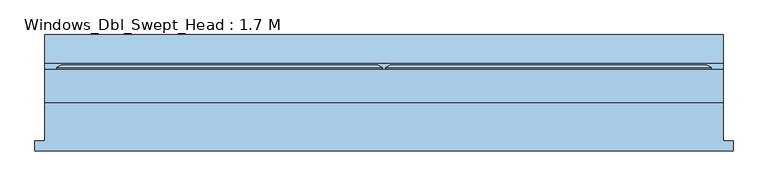
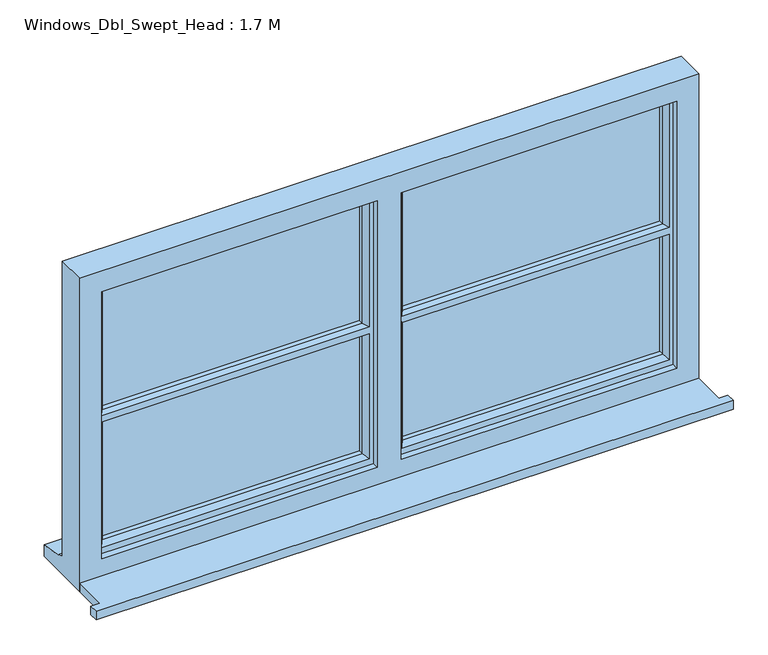
"""IFC4 building model written with IfcOpenShell, lengths in millimetres: window geometry, Windows_Dbl_Swept_Head : 1.7 M."""

from ifc_helpers import new_model, si_unit, frame, origin, place, context, project, spatial, polyline, circle_curve, outline, extrude, faceted_brep, source, transform, mapped, element, save
from ifc_brep_helpers import plane_surface, revolved_surface, advanced_brep


def windows_dbl_swept_head_1_7_m_3b36615c(model_context):
    return source(origin(), model_context, "Body", "SolidModel", [
        extrude(outline(polyline([(-1160.0, -130.8434322), (-1160.0, -105.8434322), (-1135.0, -105.8434322), (-1135.0, -10.2434322), (565.0, -10.2434322), (565.0, -105.8434322), (590.0, -105.8434322), (590.0, -130.8434322), (-1160.0, -130.8434322)])), frame((0.0, 0.0, 1200.0), z_axis=(0.0, 0.0, 1.0), x_axis=(1.0, 0.0, 0.0)), (0.0, 0.0, 1.0), 25.0),
        extrude(outline(polyline([(495.1480377, 36.7565678), (-240.0, 36.7565678), (-240.0, 60.7565678), (495.1480377, 60.7565678), (495.1480377, 36.7565678)])), frame((0.0, 0.0, 1293.0), z_axis=(0.0, 0.0, 1.0), x_axis=(1.0, 0.0, 0.0)), (0.0, 0.0, 1.0), 365.5),
        extrude(outline(polyline([(495.1480377, 36.7565678), (-240.0, 36.7565678), (-240.0, 60.7565678), (495.1480377, 60.7565678), (495.1480377, 36.7565678)])), frame((0.0, 0.0, 1674.5), z_axis=(0.0, 0.0, 1.0), x_axis=(1.0, 0.0, 0.0)), (0.0, 0.0, 1.0), 365.5),
        extrude(outline(polyline([(-330.0, 36.7565678), (-1065.0, 36.7565678), (-1065.0, 60.7565678), (-330.0, 60.7565678), (-330.0, 36.7565678)])), frame((0.0, 0.0, 1674.5), z_axis=(0.0, 0.0, 1.0), x_axis=(1.0, 0.0, 0.0)), (0.0, 0.0, 1.0), 365.5),
        extrude(outline(polyline([(-330.0, 36.7565678), (-1065.1480377, 36.7565678), (-1065.1480377, 60.7565678), (-330.0, 60.7565678), (-330.0, 36.7565678)])), frame((0.0, 0.0, 1292.8519623), z_axis=(0.0, 0.0, 1.0), x_axis=(1.0, 0.0, 0.0)), (0.0, 0.0, 1.0), 365.6480377),
        faceted_brep([(-1135.0, -10.2434322, 1200.0), (565.0, -10.2434322, 1200.0), (565.0, -10.2434322, 2110.0), (-1135.0, -10.2434322, 2110.0), (-318.0, -10.2434322, 2050.0), (-318.0, -10.2434322, 1275.0), (-1075.0, -10.2434322, 1275.0), (-1075.0, -10.2434322, 2050.0), (-252.0, -10.2434322, 2050.0), (505.0, -10.2434322, 2050.0), (505.0, -10.2434322, 1275.0), (-252.0, -10.2434322, 1275.0), (-1135.0, 72.7565678, 2110.0), (-1135.0, 72.7565678, 1251.0), (-1135.0, 87.7565678, 1249.68767), (-1135.0, 87.7565678, 1244.7449676), (-1135.0, 160.2565678, 1233.8088847), (-1135.0, 160.2565678, 1200.0), (565.0, 72.7565678, 2110.0), (565.0, 72.7565678, 1251.0), (-1095.0, 72.7565678, 2070.0), (-1095.0, 72.7565678, 1263.0), (-300.0, 72.7565678, 1263.0), (-300.0, 72.7565678, 2070.0), (-270.0, 72.7565678, 2070.0), (-270.0, 72.7565678, 1263.0), (525.0, 72.7565678, 1263.0), (525.0, 72.7565678, 2070.0), (-1095.0, 7.7565678, 2070.0), (-1095.0, 7.7565678, 1263.0), (-300.0, 7.7565678, 2070.0), (-300.0, 7.7565678, 1263.0), (-318.0, 7.7565678, 2050.0), (-1075.0, 7.7565678, 2050.0), (-1075.0, 7.7565678, 1275.0), (-318.0, 7.7565678, 1275.0), (-270.0, 7.7565678, 2070.0), (525.0, 7.7565678, 2070.0), (525.0, 7.7565678, 1263.0), (-270.0, 7.7565678, 1263.0), (505.0, 7.7565678, 2050.0), (-252.0, 7.7565678, 2050.0), (-252.0, 7.7565678, 1275.0), (505.0, 7.7565678, 1275.0), (565.0, 160.2565678, 1200.0), (565.0, 160.2565678, 1233.8088847), (565.0, 87.7565678, 1244.7449676), (565.0, 87.7565678, 1249.68767)], [[[0, 1, 2, 3], [4, 5, 6, 7], [8, 9, 10, 11]], [[0, 3, 12, 13, 14, 15, 16, 17]], [[13, 12, 18, 19], [20, 21, 22, 23], [24, 25, 26, 27]], [[21, 20, 28, 29]], [[28, 30, 31, 29], [32, 33, 34, 35]], [[36, 37, 38, 39], [40, 41, 42, 43]], [[33, 7, 6, 34]], [[12, 3, 2, 18]], [[28, 20, 23, 30]], [[27, 37, 36, 24]], [[7, 33, 32, 4]], [[40, 9, 8, 41]], [[19, 18, 2, 1, 44, 45, 46, 47]], [[27, 26, 38, 37]], [[9, 40, 43, 10]], [[23, 22, 31, 30]], [[25, 24, 36, 39]], [[41, 8, 11, 42]], [[4, 32, 35, 5]], [[44, 1, 0, 17]], [[45, 44, 17, 16]], [[46, 45, 16, 15]], [[47, 46, 15, 14]], [[19, 47, 14, 13]], [[22, 21, 29, 31]], [[26, 25, 39, 38]], [[11, 10, 43, 42]], [[35, 34, 6, 5]]]),
        advanced_brep(
        [(-280.0, 72.7565678, 2080.0), (-280.0, 78.5300705, 2080.0), (-280.0, 78.5300705, 1253.0), (-280.0, 72.7565678, 1253.0), (-270.0, 7.7565678, 2070.0), (-270.0, 72.7565678, 2070.0), (-270.0, 72.7565678, 1263.0), (-270.0, 7.7565678, 1263.0), (-230.0, 22.2494677, 2030.0), (-240.1480377, 7.7565678, 2040.1480377), (-240.1480377, 7.7565678, 1676.3519623), (-230.0, 22.2494677, 1681.5), (-240.1480377, 7.7565678, 1292.8519623), (-230.0, 22.2494677, 1303.0), (-230.0, 22.2494677, 1651.5), (-240.1480377, 7.7565678, 1656.6480377), (-230.0, 36.7565678, 2030.0), (-230.0, 36.7565678, 1681.5), (-230.0, 36.7565678, 1303.0), (-230.0, 36.7565678, 1651.5), (-240.0, 60.7565678, 2040.0), (-240.0, 36.7565678, 2040.0), (-240.0, 36.7565678, 1674.5), (-240.0, 60.7565678, 1674.5), (-240.0, 36.7565678, 1293.0), (-240.0, 60.7565678, 1293.0), (-240.0, 60.7565678, 1658.5), (-240.0, 36.7565678, 1658.5), (-230.0, 60.7565678, 1303.0), (-230.0, 78.5300705, 1303.0), (-230.0, 78.5300705, 1651.5), (-230.0, 60.7565678, 1651.5), (-230.0, 60.7565678, 1681.5), (-230.0, 78.5300705, 1681.5), (-230.0, 78.5300705, 1926.8253484), (-230.0, 60.7565678, 1926.8253484), (-247.4457548, 84.3035732, 2047.4457548), (-230.0, 78.5300705, 2030.0), (-235.0, 80.1847718, 1681.5), (-247.4457548, 84.3035732, 1669.0542452), (-247.4457548, 84.3035732, 1285.5542452), (-247.4457548, 84.3035732, 1663.9457548), (-235.0, 80.1847718, 1651.5), (-269.2153903, 84.3035732, 2069.2153903), (-269.2153903, 84.3035732, 1263.7846097), (535.0, 78.5300705, 1253.0), (535.0, 72.7565678, 1253.0), (525.0, 72.7565678, 1263.0), (525.0, 7.7565678, 1263.0), (495.1480377, 7.7565678, 1292.8519623), (485.0, 22.2494677, 1303.0), (485.0, 36.7565678, 1303.0), (495.0, 36.7565678, 1293.0), (495.0, 60.7565678, 1293.0), (485.0, 60.7565678, 1303.0), (485.0, 78.5300705, 1303.0), (502.4457548, 84.3035732, 1285.5542452), (524.2153903, 84.3035732, 1263.7846097), (535.0, 78.5300705, 2080.0), (535.0, 72.7565678, 2080.0), (525.0, 72.7565678, 2070.0), (525.0, 7.7565678, 2070.0), (495.1480377, 7.7565678, 1656.6480377), (485.0, 22.2494677, 1651.5), (495.1480377, 7.7565678, 2040.1480377), (485.0, 22.2494677, 2030.0), (485.0, 22.2494677, 1681.5), (495.1480377, 7.7565678, 1676.3519623), (485.0, 36.7565678, 1651.5), (485.0, 36.7565678, 2030.0), (485.0, 36.7565678, 1681.5), (495.0, 36.7565678, 1658.5), (495.0, 60.7565678, 1658.5), (495.0, 36.7565678, 2040.0), (495.0, 60.7565678, 2040.0), (495.0, 60.7565678, 1674.5), (495.0, 36.7565678, 1674.5), (485.0, 60.7565678, 1651.5), (485.0, 78.5300705, 1651.5), (485.0, 78.5300705, 1681.5), (485.0, 60.7565678, 1681.5), (485.0, 60.7565678, 1926.8253484), (485.0, 78.5300705, 1926.8253484), (490.0, 80.1847718, 1651.5), (502.4457548, 84.3035732, 1663.9457548), (485.0, 78.5300705, 2030.0), (502.4457548, 84.3035732, 2047.4457548), (502.4457548, 84.3035732, 1669.0542452), (490.0, 80.1847718, 1681.5), (524.2153903, 84.3035732, 2069.2153903)],
        [
            (0, 1),
            (1, 2),
            (2, 3),
            (3, 0),
            (4, 5),
            (5, 6),
            (6, 7),
            (7, 4),
            (8, 9),
            (9, 10),
            (10, 11),
            (11, 8),
            (12, 13),
            (13, 14),
            (14, 15),
            (15, 12),
            (16, 8),
            (11, 17),
            (17, 16),
            (13, 18),
            (18, 19),
            (19, 14),
            (20, 21),
            (21, 22),
            (22, 23),
            (23, 20),
            (24, 25),
            (25, 26),
            (26, 27),
            (27, 24),
            (28, 29),
            (29, 30),
            (30, 31),
            (31, 28),
            (32, 33),
            (33, 34),
            (34, 35),
            (35, 32),
            (36, 37),
            (37, 34),
            (33, 38),
            (38, 39),
            (39, 36),
            (29, 40),
            (40, 41),
            (41, 42),
            (42, 30),
            (1, 43),
            (43, 44),
            (44, 2),
            (2, 45),
            (45, 46),
            (46, 3),
            (6, 47),
            (47, 48),
            (48, 7),
            (12, 49),
            (49, 50),
            (50, 13),
            (50, 51),
            (51, 18),
            (24, 52),
            (52, 53),
            (53, 25),
            (28, 54),
            (54, 55),
            (55, 29),
            (55, 56),
            (56, 40),
            (44, 57),
            (57, 45),
            (45, 58),
            (58, 59),
            (59, 46),
            (47, 60),
            (60, 61),
            (61, 48),
            (49, 62),
            (62, 63),
            (63, 50),
            (64, 65),
            (65, 66),
            (66, 67),
            (67, 64),
            (63, 68),
            (68, 51),
            (65, 69),
            (69, 70),
            (70, 66),
            (52, 71),
            (71, 72),
            (72, 53),
            (73, 74),
            (74, 75),
            (75, 76),
            (76, 73),
            (54, 77),
            (77, 78),
            (78, 55),
            (79, 80),
            (80, 81),
            (81, 82),
            (82, 79),
            (78, 83),
            (83, 84),
            (84, 56),
            (85, 86),
            (86, 87),
            (87, 88),
            (88, 79),
            (82, 85),
            (57, 89),
            (89, 58),
            (0, 59),
            (58, 1),
            (5, 60),
            (4, 61),
            (15, 62),
            (9, 64),
            (67, 10),
            (8, 65),
            (16, 69),
            (27, 71),
            (68, 19),
            (21, 73),
            (76, 22),
            (17, 70),
            (20, 74),
            (72, 26),
            (31, 77),
            (23, 75),
            (80, 32),
            (35, 81, circle_curve(frame((127.5, 60.7565678, 1325.0), z_axis=(0.0, 1.0, 0.0), x_axis=(1.0, 0.0, 0.0)), 700.0)),
            (36, 86),
            (85, 37),
            (43, 89),
            (84, 41),
            (39, 87),
            (38, 88),
            (11, 66),
            (14, 63),
            (42, 83),
            (82, 34, circle_curve(frame((127.5, 78.5300705, 1325.0), z_axis=(0.0, -1.0, 0.0), x_axis=(1.0, 0.0, 0.0)), 700.0)),
        ],
        [
            plane_surface(frame((-280.0, 78.5300705, 2080.0), z_axis=(-1.0, 0.0, 0.0), x_axis=(0.0, 0.0, -1.0))),
            plane_surface(frame((-270.0, 72.7565678, 2070.0), z_axis=(-1.0, 0.0, 0.0), x_axis=(0.0, 0.0, -1.0))),
            plane_surface(frame((-240.1480377, 7.7565678, 2040.1480377), z_axis=(0.8191520442889492, -0.5735764363511071, 0.0), x_axis=(0.0, 0.0, -1.0))),
            plane_surface(frame((-230.0, 22.2494677, 2030.0), z_axis=(1.0, 0.0, 0.0), x_axis=(0.0, 0.0, -1.0))),
            plane_surface(frame((-240.0, 36.7565678, 2040.0), z_axis=(1.0, 0.0, 0.0), x_axis=(0.0, 0.0, -1.0))),
            plane_surface(frame((-230.0, 60.7565678, 2030.0), z_axis=(1.0, 0.0, 0.0), x_axis=(0.0, 0.0, -1.0))),
            plane_surface(frame((-230.0, 78.5300705, 2030.0), z_axis=(0.31418232948755237, 0.9493626619147053, 0.0), x_axis=(0.0, 0.0, -1.0))),
            plane_surface(frame((-269.2153903, 84.3035732, 2069.2153903), z_axis=(-0.47196942945730275, 0.8816149146071363, 0.0), x_axis=(0.0, 0.0, -1.0))),
            plane_surface(frame((-280.0, 78.5300705, 1253.0), z_axis=(0.0, 0.0, -1.0), x_axis=(1.0, 0.0, 0.0))),
            plane_surface(frame((-270.0, 72.7565678, 1263.0), z_axis=(0.0, 0.0, -1.0), x_axis=(1.0, 0.0, 0.0))),
            plane_surface(frame((-240.1480377, 7.7565678, 1292.8519623), z_axis=(0.0, -0.5735764363511044, 0.819152044288951), x_axis=(1.0, 0.0, 0.0))),
            plane_surface(frame((-230.0, 22.2494677, 1303.0), z_axis=(0.0, 0.0, 1.0), x_axis=(1.0, 0.0, 0.0))),
            plane_surface(frame((-240.0, 36.7565678, 1293.0), z_axis=(0.0, 0.0, 1.0), x_axis=(1.0, 0.0, 0.0))),
            plane_surface(frame((-230.0, 60.7565678, 1303.0), z_axis=(0.0, 0.0, 1.0), x_axis=(1.0, 0.0, 0.0))),
            plane_surface(frame((-230.0, 78.5300705, 1303.0), z_axis=(0.0, 0.9493626619147063, 0.31418232948754926), x_axis=(1.0, 0.0, 0.0))),
            plane_surface(frame((-269.2153903, 84.3035732, 1263.7846097), z_axis=(0.0, 0.8816149146071347, -0.47196942945730563), x_axis=(1.0, 0.0, 0.0))),
            plane_surface(frame((535.0, 78.5300705, 1253.0), z_axis=(1.0, 0.0, 0.0), x_axis=(0.0, 0.0, 1.0))),
            plane_surface(frame((525.0, 72.7565678, 1263.0), z_axis=(1.0, 0.0, 0.0), x_axis=(0.0, 0.0, 1.0))),
            plane_surface(frame((495.1480377, 7.7565678, 1292.8519623), z_axis=(-0.8191520442889529, -0.5735764363511018, 0.0), x_axis=(0.0, 0.0, 1.0))),
            plane_surface(frame((485.0, 22.2494677, 1303.0), z_axis=(-1.0, 0.0, 0.0), x_axis=(0.0, 0.0, 1.0))),
            plane_surface(frame((495.0, 36.7565678, 1293.0), z_axis=(-1.0, 0.0, 0.0), x_axis=(0.0, 0.0, 1.0))),
            plane_surface(frame((485.0, 60.7565678, 1303.0), z_axis=(-1.0, 0.0, 0.0), x_axis=(0.0, 0.0, 1.0))),
            plane_surface(frame((485.0, 78.5300705, 1303.0), z_axis=(-0.3141823294875462, 0.9493626619147074, 0.0), x_axis=(0.0, 0.0, 1.0))),
            plane_surface(frame((524.2153903, 84.3035732, 1263.7846097), z_axis=(0.4719694294573085, 0.8816149146071331, 0.0), x_axis=(0.0, 0.0, 1.0))),
            plane_surface(frame((535.0, 78.5300705, 2080.0), z_axis=(0.0, 0.0, 1.0), x_axis=(-1.0, 0.0, 0.0))),
            plane_surface(frame((535.0, 72.7565678, 2080.0), z_axis=(0.0, -1.0, 0.0), x_axis=(-1.0, 0.0, 0.0))),
            plane_surface(frame((525.0, 72.7565678, 2070.0), z_axis=(0.0, 0.0, 1.0), x_axis=(-1.0, 0.0, 0.0))),
            plane_surface(frame((525.0, 7.7565678, 2070.0), z_axis=(0.0, -1.0, 0.0), x_axis=(-1.0, 0.0, 0.0))),
            plane_surface(frame((495.1480377, 7.7565678, 2040.1480377), z_axis=(0.0, -0.5735764363511044, -0.819152044288951), x_axis=(-1.0, 0.0, 0.0))),
            plane_surface(frame((485.0, 22.2494677, 2030.0), z_axis=(0.0, 0.0, -1.0), x_axis=(-1.0, 0.0, 0.0))),
            plane_surface(frame((485.0, 36.7565678, 2030.0), z_axis=(0.0, 1.0, 0.0), x_axis=(-1.0, 0.0, 0.0))),
            plane_surface(frame((495.0, 36.7565678, 2040.0), z_axis=(0.0, 0.0, -1.0), x_axis=(-1.0, 0.0, 0.0))),
            plane_surface(frame((495.0, 60.7565678, 2040.0), z_axis=(0.0, -1.0, 0.0), x_axis=(-1.0, 0.0, 0.0))),
            plane_surface(frame((485.0, 78.5300705, 2030.0), z_axis=(0.0, 0.9493626619147064, -0.3141823294875493), x_axis=(-1.0, 0.0, 0.0))),
            plane_surface(frame((502.4457548, 84.3035732, 2047.4457548), z_axis=(0.0, 1.0, 0.0), x_axis=(-1.0, 0.0, 0.0))),
            plane_surface(frame((524.2153903, 84.3035732, 2069.2153903), z_axis=(0.0, 0.8816149146071347, 0.47196942945730563), x_axis=(-1.0, 0.0, 0.0))),
            plane_surface(frame((502.4457548, 84.3035732, 1669.0542452), z_axis=(0.0, 0.9493626619145938, 0.3141823294878896), x_axis=(-1.0, 0.0, 0.0))),
            plane_surface(frame((502.4457548, 80.1847718, 1681.5), z_axis=(0.0, 0.0, 1.0), x_axis=(-1.0, 0.0, 0.0))),
            plane_surface(frame((502.4457548, 60.7565678, 1674.5), z_axis=(0.0, 0.0, 1.0), x_axis=(-1.0, 0.0, 0.0))),
            plane_surface(frame((502.4457548, 36.7565678, 1681.5), z_axis=(0.0, 0.0, 1.0), x_axis=(-1.0, 0.0, 0.0))),
            plane_surface(frame((502.4457548, 22.2494677, 1681.5), z_axis=(0.0, -0.33472142672711697, 0.9423171262848634), x_axis=(-1.0, 0.0, 0.0))),
            plane_surface(frame((502.4457548, 7.7565678, 1656.6480377), z_axis=(0.0, -0.33472142672499106, -0.9423171262856186), x_axis=(-1.0, 0.0, 0.0))),
            plane_surface(frame((502.4457548, 22.2494677, 1651.5), z_axis=(0.0, 0.0, -1.0), x_axis=(-1.0, 0.0, 0.0))),
            plane_surface(frame((502.4457548, 36.7565678, 1658.5), z_axis=(0.0, 0.0, -1.0), x_axis=(-1.0, 0.0, 0.0))),
            plane_surface(frame((502.4457548, 60.7565678, 1651.5), z_axis=(0.0, 0.0, -1.0), x_axis=(-1.0, 0.0, 0.0))),
            plane_surface(frame((502.4457548, 80.1847718, 1651.5), z_axis=(0.0, 0.9493626619148547, -0.31418232948710106), x_axis=(-1.0, 0.0, 0.0))),
            plane_surface(frame((-230.0, 78.5300705, 2030.0), z_axis=(0.0, 1.0, 0.0), x_axis=(0.0, 0.0, 1.0))),
            revolved_surface(polyline([(827.5, 78.5300705, 1325.0), (827.5, 60.7565678, 1325.0)]), (127.5, 78.5300705, 1325.0), (0.0, 1.0, 0.0)),
        ],
        [
            (0, [[1, 2, 3, 4]]),
            (1, [[5, 6, 7, 8]]),
            (2, [[9, 10, 11, 12]]),
            (2, [[13, 14, 15, 16]]),
            (3, [[17, -12, 18, 19]]),
            (3, [[20, 21, 22, -14]]),
            (4, [[23, 24, 25, 26]]),
            (4, [[27, 28, 29, 30]]),
            (5, [[31, 32, 33, 34]]),
            (5, [[35, 36, 37, 38]]),
            (6, [[39, 40, -36, 41, 42, 43]]),
            (6, [[44, 45, 46, 47, -32]]),
            (7, [[-2, 48, 49, 50]]),
            (8, [[-3, 51, 52, 53]]),
            (9, [[-7, 54, 55, 56]]),
            (10, [[-13, 57, 58, 59]]),
            (11, [[-20, -59, 60, 61]]),
            (12, [[-27, 62, 63, 64]]),
            (13, [[-31, 65, 66, 67]]),
            (14, [[-44, -67, 68, 69]]),
            (15, [[-50, 70, 71, -51]]),
            (16, [[-52, 72, 73, 74]]),
            (17, [[-55, 75, 76, 77]]),
            (18, [[-58, 78, 79, 80]]),
            (18, [[81, 82, 83, 84]]),
            (19, [[-60, -80, 85, 86]]),
            (19, [[87, 88, 89, -82]]),
            (20, [[-63, 90, 91, 92]]),
            (20, [[93, 94, 95, 96]]),
            (21, [[-66, 97, 98, 99]]),
            (21, [[100, 101, 102, 103]]),
            (22, [[-68, -99, 104, 105, 106]]),
            (22, [[107, 108, 109, 110, -103, 111]]),
            (23, [[-71, 112, 113, -72]]),
            (24, [[-1, 114, -73, 115]]),
            (25, [[-4, -53, -74, -114], [-6, 116, -75, -54]]),
            (26, [[-5, 117, -76, -116]]),
            (27, [[-8, -56, -77, -117], [-57, -16, 118, -78], [119, -84, 120, -10]]),
            (28, [[-9, 121, -81, -119]]),
            (29, [[-17, 122, -87, -121]]),
            (30, [[-62, -30, 123, -90], [-61, -86, 124, -21]]),
            (30, [[125, -96, 126, -24], [-122, -19, 127, -88]]),
            (31, [[-23, 128, -93, -125]]),
            (32, [[-64, -92, 129, -28], [-65, -34, 130, -97]]),
            (32, [[-128, -26, 131, -94], [132, -38, 133, -101]]),
            (33, [[-39, 134, -107, 135]]),
            (34, [[-49, 136, -112, -70], [-69, -106, 137, -45], [-134, -43, 138, -108]]),
            (35, [[-48, -115, -113, -136]]),
            (36, [[-138, -42, 139, -109]]),
            (37, [[-132, -100, -110, -139, -41, -35]]),
            (38, [[-25, -126, -95, -131]]),
            (39, [[140, -89, -127, -18]]),
            (40, [[-120, -83, -140, -11]]),
            (41, [[-118, -15, 141, -79]]),
            (42, [[-141, -22, -124, -85]]),
            (43, [[-29, -129, -91, -123]]),
            (44, [[-130, -33, -47, 142, -104, -98]]),
            (45, [[-137, -105, -142, -46]]),
            (46, [[143, -40, -135, -111]]),
            (47, [[-133, -37, -143, -102]]),
        ],
    ),
        advanced_brep(
        [(-330.0, 60.7565678, 2040.0), (-1065.0, 60.7565678, 2040.0), (-1065.0, 60.7565678, 1674.5), (-330.0, 60.7565678, 1674.5), (-1055.0, 60.7565678, 1926.8253484), (-340.0, 60.7565678, 1926.8253484), (-340.0, 60.7565678, 1681.5), (-1055.0, 60.7565678, 1681.5), (-1065.0, 60.7565678, 1293.0), (-330.0, 60.7565678, 1293.0), (-330.0, 60.7565678, 1658.5), (-1065.0, 60.7565678, 1658.5), (-340.0, 60.7565678, 1303.0), (-1055.0, 60.7565678, 1303.0), (-1055.0, 60.7565678, 1651.5), (-340.0, 60.7565678, 1651.5), (-1105.0, 72.7565678, 2080.0), (-1105.0, 78.5300705, 2080.0), (-1105.0, 78.5300705, 1253.0), (-1105.0, 72.7565678, 1253.0), (-1095.0, 7.7565678, 2070.0), (-1095.0, 72.7565678, 2070.0), (-1095.0, 72.7565678, 1263.0), (-1095.0, 7.7565678, 1263.0), (-1055.0, 22.2494677, 2030.0), (-1065.1480377, 7.7565678, 2040.1480377), (-1065.1480377, 7.7565678, 1676.3519623), (-1055.0, 22.2494677, 1681.5), (-1065.1480377, 7.7565678, 1292.8519623), (-1055.0, 22.2494677, 1303.0), (-1055.0, 22.2494677, 1651.5), (-1065.1480377, 7.7565678, 1656.6480377), (-1055.0, 36.7565678, 2030.0), (-1055.0, 36.7565678, 1681.5), (-1055.0, 36.7565678, 1303.0), (-1055.0, 36.7565678, 1651.5), (-1065.0, 36.7565678, 2040.0), (-1065.0, 36.7565678, 1674.5), (-1065.0, 36.7565678, 1293.0), (-1065.0, 36.7565678, 1658.5), (-1055.0, 78.5300705, 1303.0), (-1055.0, 78.5300705, 1651.5), (-1055.0, 78.5300705, 1681.5), (-1055.0, 78.5300705, 1926.8253484), (-1072.4457548, 84.3035732, 2047.4457548), (-1055.0, 78.5300705, 2030.0), (-1060.0, 80.1847718, 1681.5), (-1072.4457548, 84.3035732, 1669.0542452), (-1072.4457548, 84.3035732, 1285.5542452), (-1072.4457548, 84.3035732, 1663.9457548), (-1060.0, 80.1847718, 1651.5), (-1094.2153903, 84.3035732, 2069.2153903), (-1094.2153903, 84.3035732, 1263.7846097), (-290.0, 78.5300705, 1253.0), (-290.0, 72.7565678, 1253.0), (-300.0, 72.7565678, 1263.0), (-300.0, 7.7565678, 1263.0), (-329.8519623, 7.7565678, 1292.8519623), (-340.0, 22.2494677, 1303.0), (-340.0, 36.7565678, 1303.0), (-330.0, 36.7565678, 1293.0), (-340.0, 78.5300705, 1303.0), (-322.5542452, 84.3035732, 1285.5542452), (-300.7846097, 84.3035732, 1263.7846097), (-290.0, 78.5300705, 2080.0), (-290.0, 72.7565678, 2080.0), (-300.0, 72.7565678, 2070.0), (-300.0, 7.7565678, 2070.0), (-329.8519623, 7.7565678, 1656.6480377), (-340.0, 22.2494677, 1651.5), (-329.8519623, 7.7565678, 2040.1480377), (-340.0, 22.2494677, 2030.0), (-340.0, 22.2494677, 1681.5), (-329.8519623, 7.7565678, 1676.3519623), (-340.0, 36.7565678, 1651.5), (-340.0, 36.7565678, 2030.0), (-340.0, 36.7565678, 1681.5), (-330.0, 36.7565678, 1658.5), (-330.0, 36.7565678, 2040.0), (-330.0, 36.7565678, 1674.5), (-340.0, 78.5300705, 1651.5), (-340.0, 78.5300705, 1681.5), (-340.0, 78.5300705, 1926.8253484), (-335.0, 80.1847718, 1651.5), (-322.5542452, 84.3035732, 1663.9457548), (-340.0, 78.5300705, 2030.0), (-322.5542452, 84.3035732, 2047.4457548), (-322.5542452, 84.3035732, 1669.0542452), (-335.0, 80.1847718, 1681.5), (-300.7846097, 84.3035732, 2069.2153903)],
        [
            (0, 1),
            (1, 2),
            (2, 3),
            (3, 0),
            (4, 5, circle_curve(frame((-697.5, 60.7565678, 1325.0), z_axis=(0.0, 1.0, 0.0), x_axis=(1.0, 0.0, 0.0)), 700.0)),
            (5, 6),
            (6, 7),
            (7, 4),
            (8, 9),
            (9, 10),
            (10, 11),
            (11, 8),
            (12, 13),
            (13, 14),
            (14, 15),
            (15, 12),
            (16, 17),
            (17, 18),
            (18, 19),
            (19, 16),
            (20, 21),
            (21, 22),
            (22, 23),
            (23, 20),
            (24, 25),
            (25, 26),
            (26, 27),
            (27, 24),
            (28, 29),
            (29, 30),
            (30, 31),
            (31, 28),
            (32, 24),
            (27, 33),
            (33, 32),
            (29, 34),
            (34, 35),
            (35, 30),
            (1, 36),
            (36, 37),
            (37, 2),
            (38, 8),
            (11, 39),
            (39, 38),
            (13, 40),
            (40, 41),
            (41, 14),
            (7, 42),
            (42, 43),
            (43, 4),
            (44, 45),
            (45, 43),
            (42, 46),
            (46, 47),
            (47, 44),
            (40, 48),
            (48, 49),
            (49, 50),
            (50, 41),
            (17, 51),
            (51, 52),
            (52, 18),
            (18, 53),
            (53, 54),
            (54, 19),
            (22, 55),
            (55, 56),
            (56, 23),
            (28, 57),
            (57, 58),
            (58, 29),
            (58, 59),
            (59, 34),
            (38, 60),
            (60, 9),
            (12, 61),
            (61, 40),
            (61, 62),
            (62, 48),
            (52, 63),
            (63, 53),
            (53, 64),
            (64, 65),
            (65, 54),
            (55, 66),
            (66, 67),
            (67, 56),
            (57, 68),
            (68, 69),
            (69, 58),
            (70, 71),
            (71, 72),
            (72, 73),
            (73, 70),
            (69, 74),
            (74, 59),
            (71, 75),
            (75, 76),
            (76, 72),
            (60, 77),
            (77, 10),
            (78, 0),
            (3, 79),
            (79, 78),
            (15, 80),
            (80, 61),
            (81, 6),
            (5, 82),
            (82, 81),
            (80, 83),
            (83, 84),
            (84, 62),
            (85, 86),
            (86, 87),
            (87, 88),
            (88, 81),
            (82, 85),
            (63, 89),
            (89, 64),
            (16, 65),
            (64, 17),
            (21, 66),
            (20, 67),
            (31, 68),
            (25, 70),
            (73, 26),
            (24, 71),
            (32, 75),
            (39, 77),
            (74, 35),
            (36, 78),
            (79, 37),
            (33, 76),
            (44, 86),
            (85, 45),
            (51, 89),
            (84, 49),
            (47, 87),
            (46, 88),
            (83, 50),
            (69, 30),
            (72, 27),
            (82, 43, circle_curve(frame((-697.5, 78.5300705, 1325.0), z_axis=(0.0, -1.0, 0.0), x_axis=(1.0, 0.0, 0.0)), 700.0)),
        ],
        [
            plane_surface(frame((495.0, 60.7565678, 2040.0), z_axis=(0.0, -1.0, 0.0), x_axis=(-1.0, 0.0, 0.0))),
            plane_surface(frame((-1105.0, 78.5300705, 2080.0), z_axis=(-1.0, 0.0, 0.0), x_axis=(0.0, 0.0, -1.0))),
            plane_surface(frame((-1095.0, 72.7565678, 2070.0), z_axis=(-1.0, 0.0, 0.0), x_axis=(0.0, 0.0, -1.0))),
            plane_surface(frame((-1065.1480377, 7.7565678, 2040.1480377), z_axis=(0.8191520442889492, -0.5735764363511071, 0.0), x_axis=(0.0, 0.0, -1.0))),
            plane_surface(frame((-1055.0, 22.2494677, 2030.0), z_axis=(1.0, 0.0, 0.0), x_axis=(0.0, 0.0, -1.0))),
            plane_surface(frame((-1065.0, 36.7565678, 2040.0), z_axis=(1.0, 0.0, 0.0), x_axis=(0.0, 0.0, -1.0))),
            plane_surface(frame((-1055.0, 60.7565678, 2030.0), z_axis=(1.0, 0.0, 0.0), x_axis=(0.0, 0.0, -1.0))),
            plane_surface(frame((-1055.0, 78.5300705, 2030.0), z_axis=(0.31418232948755237, 0.9493626619147053, 0.0), x_axis=(0.0, 0.0, -1.0))),
            plane_surface(frame((-1094.2153903, 84.3035732, 2069.2153903), z_axis=(-0.47196942945730275, 0.8816149146071363, 0.0), x_axis=(0.0, 0.0, -1.0))),
            plane_surface(frame((-1105.0, 78.5300705, 1253.0), z_axis=(0.0, 0.0, -1.0), x_axis=(1.0, 0.0, 0.0))),
            plane_surface(frame((-1095.0, 72.7565678, 1263.0), z_axis=(0.0, 0.0, -1.0), x_axis=(1.0, 0.0, 0.0))),
            plane_surface(frame((-1065.1480377, 7.7565678, 1292.8519623), z_axis=(0.0, -0.5735764363511044, 0.819152044288951), x_axis=(1.0, 0.0, 0.0))),
            plane_surface(frame((-1055.0, 22.2494677, 1303.0), z_axis=(0.0, 0.0, 1.0), x_axis=(1.0, 0.0, 0.0))),
            plane_surface(frame((-1065.0, 36.7565678, 1293.0), z_axis=(0.0, 0.0, 1.0), x_axis=(1.0, 0.0, 0.0))),
            plane_surface(frame((-1055.0, 60.7565678, 1303.0), z_axis=(0.0, 0.0, 1.0), x_axis=(1.0, 0.0, 0.0))),
            plane_surface(frame((-1055.0, 78.5300705, 1303.0), z_axis=(0.0, 0.9493626619147063, 0.31418232948754926), x_axis=(1.0, 0.0, 0.0))),
            plane_surface(frame((-1094.2153903, 84.3035732, 1263.7846097), z_axis=(0.0, 0.8816149146071347, -0.47196942945730563), x_axis=(1.0, 0.0, 0.0))),
            plane_surface(frame((-290.0, 78.5300705, 1253.0), z_axis=(1.0, 0.0, 0.0), x_axis=(0.0, 0.0, 1.0))),
            plane_surface(frame((-300.0, 72.7565678, 1263.0), z_axis=(1.0, 0.0, 0.0), x_axis=(0.0, 0.0, 1.0))),
            plane_surface(frame((-329.8519623, 7.7565678, 1292.8519623), z_axis=(-0.8191520442889529, -0.5735764363511018, 0.0), x_axis=(0.0, 0.0, 1.0))),
            plane_surface(frame((-340.0, 22.2494677, 1303.0), z_axis=(-1.0, 0.0, 0.0), x_axis=(0.0, 0.0, 1.0))),
            plane_surface(frame((-330.0, 36.7565678, 1293.0), z_axis=(-1.0, 0.0, 0.0), x_axis=(0.0, 0.0, 1.0))),
            plane_surface(frame((-340.0, 60.7565678, 1303.0), z_axis=(-1.0, 0.0, 0.0), x_axis=(0.0, 0.0, 1.0))),
            plane_surface(frame((-340.0, 78.5300705, 1303.0), z_axis=(-0.3141823294875462, 0.9493626619147074, 0.0), x_axis=(0.0, 0.0, 1.0))),
            plane_surface(frame((-300.7846097, 84.3035732, 1263.7846097), z_axis=(0.4719694294573085, 0.8816149146071331, 0.0), x_axis=(0.0, 0.0, 1.0))),
            plane_surface(frame((-290.0, 78.5300705, 2080.0), z_axis=(0.0, 0.0, 1.0), x_axis=(-1.0, 0.0, 0.0))),
            plane_surface(frame((-290.0, 72.7565678, 2080.0), z_axis=(0.0, -1.0, 0.0), x_axis=(-1.0, 0.0, 0.0))),
            plane_surface(frame((-300.0, 72.7565678, 2070.0), z_axis=(0.0, 0.0, 1.0), x_axis=(-1.0, 0.0, 0.0))),
            plane_surface(frame((-300.0, 7.7565678, 2070.0), z_axis=(0.0, -1.0, 0.0), x_axis=(-1.0, 0.0, 0.0))),
            plane_surface(frame((-329.8519623, 7.7565678, 2040.1480377), z_axis=(0.0, -0.5735764363511044, -0.819152044288951), x_axis=(-1.0, 0.0, 0.0))),
            plane_surface(frame((-340.0, 22.2494677, 2030.0), z_axis=(0.0, 0.0, -1.0), x_axis=(-1.0, 0.0, 0.0))),
            plane_surface(frame((-340.0, 36.7565678, 2030.0), z_axis=(0.0, 1.0, 0.0), x_axis=(-1.0, 0.0, 0.0))),
            plane_surface(frame((-330.0, 36.7565678, 2040.0), z_axis=(0.0, 0.0, -1.0), x_axis=(-1.0, 0.0, 0.0))),
            plane_surface(frame((-340.0, 78.5300705, 2030.0), z_axis=(0.0, 0.9493626619147064, -0.3141823294875493), x_axis=(-1.0, 0.0, 0.0))),
            plane_surface(frame((-322.5542452, 84.3035732, 2047.4457548), z_axis=(0.0, 1.0, 0.0), x_axis=(-1.0, 0.0, 0.0))),
            plane_surface(frame((-300.7846097, 84.3035732, 2069.2153903), z_axis=(0.0, 0.8816149146071347, 0.47196942945730563), x_axis=(-1.0, 0.0, 0.0))),
            plane_surface(frame((-1072.4457548, 80.1847718, 1681.5), z_axis=(0.0, 0.9493626619144715, 0.31418232948825914), x_axis=(1.0, 0.0, 0.0))),
            plane_surface(frame((-1072.4457548, 84.3035732, 1663.9457548), z_axis=(0.0, 0.949362661914977, -0.3141823294867314), x_axis=(1.0, 0.0, 0.0))),
            plane_surface(frame((-1072.4457548, 80.1847718, 1651.5), z_axis=(0.0, 0.0, -1.0), x_axis=(1.0, 0.0, 0.0))),
            plane_surface(frame((-1072.4457548, 60.7565678, 1658.5), z_axis=(0.0, 0.0, -1.0), x_axis=(1.0, 0.0, 0.0))),
            plane_surface(frame((-1072.4457548, 36.7565678, 1651.5), z_axis=(0.0, 0.0, -1.0), x_axis=(1.0, 0.0, 0.0))),
            plane_surface(frame((-1072.4457548, 22.2494677, 1651.5), z_axis=(0.0, -0.3347214267259168, -0.9423171262852897), x_axis=(1.0, 0.0, 0.0))),
            plane_surface(frame((-1072.4457548, 7.7565678, 1676.3519623), z_axis=(0.0, -0.33472142672616695, 0.9423171262852009), x_axis=(1.0, 0.0, 0.0))),
            plane_surface(frame((-1072.4457548, 22.2494677, 1681.5), z_axis=(0.0, 0.0, 1.0), x_axis=(1.0, 0.0, 0.0))),
            plane_surface(frame((-1072.4457548, 36.7565678, 1674.5), z_axis=(0.0, 0.0, 1.0), x_axis=(1.0, 0.0, 0.0))),
            plane_surface(frame((-1072.4457548, 60.7565678, 1681.5), z_axis=(0.0, 0.0, 1.0), x_axis=(1.0, 0.0, 0.0))),
            plane_surface(frame((-230.0, 78.5300705, 2030.0), z_axis=(0.0, 1.0, 0.0), x_axis=(0.0, 0.0, 1.0))),
            revolved_surface(polyline([(2.5, 78.5300705, 1325.0), (2.5, 60.7565678, 1325.0)]), (-697.5, 72.7565678, 1325.0), (0.0, 1.0, 0.0)),
        ],
        [
            (0, [[1, 2, 3, 4], [5, 6, 7, 8]]),
            (0, [[9, 10, 11, 12], [13, 14, 15, 16]]),
            (1, [[17, 18, 19, 20]]),
            (2, [[21, 22, 23, 24]]),
            (3, [[25, 26, 27, 28]]),
            (3, [[29, 30, 31, 32]]),
            (4, [[33, -28, 34, 35]]),
            (4, [[36, 37, 38, -30]]),
            (5, [[39, 40, 41, -2]]),
            (5, [[42, -12, 43, 44]]),
            (6, [[45, 46, 47, -14]]),
            (6, [[48, 49, 50, -8]]),
            (7, [[51, 52, -49, 53, 54, 55]]),
            (7, [[56, 57, 58, 59, -46]]),
            (8, [[-18, 60, 61, 62]]),
            (9, [[-19, 63, 64, 65]]),
            (10, [[-23, 66, 67, 68]]),
            (11, [[-29, 69, 70, 71]]),
            (12, [[-36, -71, 72, 73]]),
            (13, [[-42, 74, 75, -9]]),
            (14, [[-45, -13, 76, 77]]),
            (15, [[-56, -77, 78, 79]]),
            (16, [[-62, 80, 81, -63]]),
            (17, [[-64, 82, 83, 84]]),
            (18, [[-67, 85, 86, 87]]),
            (19, [[-70, 88, 89, 90]]),
            (19, [[91, 92, 93, 94]]),
            (20, [[-72, -90, 95, 96]]),
            (20, [[97, 98, 99, -92]]),
            (21, [[-75, 100, 101, -10]]),
            (21, [[102, -4, 103, 104]]),
            (22, [[-76, -16, 105, 106]]),
            (22, [[107, -6, 108, 109]]),
            (23, [[-78, -106, 110, 111, 112]]),
            (23, [[113, 114, 115, 116, -109, 117]]),
            (24, [[-81, 118, 119, -82]]),
            (25, [[-17, 120, -83, 121]]),
            (26, [[-20, -65, -84, -120], [-22, 122, -85, -66]]),
            (27, [[-21, 123, -86, -122]]),
            (28, [[-24, -68, -87, -123], [-69, -32, 124, -88], [125, -94, 126, -26]]),
            (29, [[-25, 127, -91, -125]]),
            (30, [[-33, 128, -97, -127]]),
            (31, [[-74, -44, 129, -100], [-73, -96, 130, -37]]),
            (31, [[131, -104, 132, -40], [-128, -35, 133, -98]]),
            (32, [[-39, -1, -102, -131]]),
            (33, [[-51, 134, -113, 135]]),
            (34, [[-61, 136, -118, -80], [-79, -112, 137, -57], [-134, -55, 138, -114]]),
            (35, [[-60, -121, -119, -136]]),
            (36, [[-138, -54, 139, -115]]),
            (37, [[-137, -111, 140, -58]]),
            (38, [[-15, -47, -59, -140, -110, -105]]),
            (39, [[-43, -11, -101, -129]]),
            (40, [[141, -38, -130, -95]]),
            (41, [[-124, -31, -141, -89]]),
            (42, [[-126, -93, 142, -27]]),
            (43, [[-142, -99, -133, -34]]),
            (44, [[-41, -132, -103, -3]]),
            (45, [[-7, -107, -116, -139, -53, -48]]),
            (46, [[143, -52, -135, -117]]),
            (47, [[-5, -50, -143, -108]]),
        ],
    ),
    ])


if __name__ == "__main__":
    model = new_model("IFC4")
    model_context = context("Model", 3, world=origin())
    ifc_project = project(units=[si_unit("LENGTHUNIT", "METRE", prefix="MILLI")], contexts=[model_context])
    site = spatial("IfcSite", under=ifc_project)
    building = spatial("IfcBuilding", under=site)
    placement = place(None, origin())
    windows_dbl_swept_head_1_7_m_shape = windows_dbl_swept_head_1_7_m_3b36615c(model_context)
    element("IfcWindow", 1, ObjectType="Windows_Dbl_Swept_Head : 1.7 M", at=placement, inside=building, context=model_context, shape_type="MappedRepresentation", body=[
        mapped(windows_dbl_swept_head_1_7_m_shape, transform((0.0, 0.0, 0.0), x_axis=(1.0, 0.0, 0.0), y_axis=(0.0, 1.0, 0.0), z_axis=(0.0, 0.0, 1.0))),
    ])
    save(model, "model.ifc")

# Revit data of these elements
# Type "Windows_Dbl_Swept_Head : 1.7 M"
#   Type Mark = "68"
#   Operation = "DoublePanelVertical"
#   Construction Type Id = "GSP4R"
#   Manufacturer = "Revit"
#   Keynote = "L10"
#   Analytic Construction = "1/8 in Pilkington single glazing"
#   Wrap Layers (Ext) from Ext = 0.1025 m
#   Wrap Layers (Int) from Ext = 0.1775 m
#   Window Board Projection = 0.025 m
#   Window Board Extension = 0.025 m
#   Visual Light Transmittance = 0.9
#   Solar Heat Gain Coefficient = 0.78
#   Rough Width = 1.7 m
#   Rough Height = 0.91 m
#   Radius - Swept Head = 0.7 m
#   Height = 0.91 m
#   Width = 1.7 m
#   Heat Transfer Coefficient (U) = 3.6886 W/(m²·K)
#   Glazing Thickness = 0.024 m
#   FrameOffset - External = 0.05 m
#   Frame Depth = 0.065 m
#   Default Head Height = 2.11 m
#   Cill Depth = 0.0875 m
#   Cavity Closer Width = 0.05 m
#   Cavity Closer Offset from Ext = 0.1025 m
#   Cavity Closer Depth = 0.085 m
#   Vis - Cavity Closers = yes
#   Define Thermal Properties by = 1
#   Material Trim = Window Frame
#   Material Glass = Glass
#   Material Frame = Window Frame
#   Wall Closure = (empty or 0)
# Element 1 (IfcWindow, "Windows_Dbl_Swept_Head : 1.7 M")
#   Materials on its faces: "Window Frame", "Glass"
# Materials
#   "Window Frame": colour RGB 249 249 249, transparency 0, Keynote = "L10", Cost = 0
#   "Glass": class "Glass", colour RGB 0 128 192, transparency 0.9, Description = "Soda Lime Glass", Cost = 0
